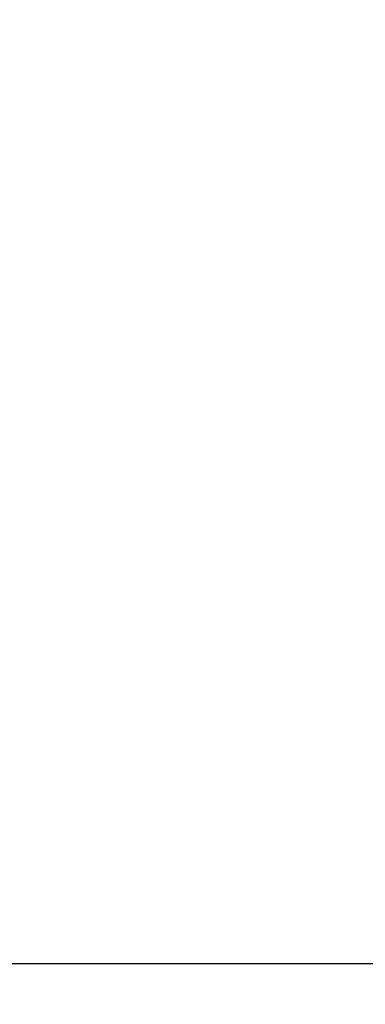
# Model space of a CAD drawing. Units: millimetres. Extents: x 0 to 2267, y 0 to 1823.
# Tile 8 of 256: x 1482.26 to 1490.3, y 1116.48 to 1139.36. Entities that reach past the tile are written whole.
import ezdxf

# ---------------------------------------------------------------- set-up
doc = ezdxf.new("R2010")
doc.units = ezdxf.units.MM
doc.header["$MEASUREMENT"] = 0
doc.layers.add('M-DIMS', color=2, linetype='Continuous', lineweight=25)
doc.layers.add('M-HATC', color=252, linetype='Continuous', lineweight=18)
doc.styles.get("Standard").update_dxf_attribs({"font": 'arial.ttf'})
doc.dimstyles.get("Standard").update_dxf_attribs({"dimtxt": 7, "dimasz": 4, "dimexe": 0.18, "dimexo": 0.0625, "dimgap": 0.09, "dimtad": 0, "dimdec": 0, "dimzin": 0, "dimdsep": 46, "dimtxsty": 'Standard', "dimcen": 0.09, "dimadec": 0, "dimazin": 0, "dimtfac": 1, "dimtdec": 0, "dimtofl": 0, "dimtmove": 0, "dimatfit": 3, "dimfxl": 1, "dimtolj": 1, "dimtzin": 0, "dimarcsym": 0})

# ---------------------------------------------------------------- blocks, each defined once
blk = doc.blocks.new('*D9')
at = {"layer": 'Defpoints', "color": 0, "transparency": 16777216}
for p in [(1332.087, 1117.417), (1505.929, 1117.417), (1505.929, 1077.417)]:
    blk.add_point(p, dxfattribs=at)
at = {"layer": 'M-DIMS', "color": 0, "lineweight": -2, "transparency": 16777216}
for p, q in [((1505.866, 1117.417), (1331.907, 1117.417)), ((1332.087, 1113.417), (1332.087, 1102.65)), ((1332.087, 1081.417), (1332.087, 1092.184)), ((1505.866, 1077.417), (1331.907, 1077.417))]:
    blk.add_line(p, q, dxfattribs=at)
at = {"layer": 'M-DIMS', "color": 0, "transparency": 16777216}
for points in [[(1331.42, 1113.417), (1332.753, 1113.417), (1332.087, 1117.417)], [(1331.42, 1081.417), (1332.753, 1081.417), (1332.087, 1077.417)]]:
    blk.add_solid(points, dxfattribs=at)
at = {"layer": 'M-DIMS', "color": 0, "transparency": 16777216, "insert": (1332.087, 1097.417), "char_height": 7, "attachment_point": 5, "rotation": 90}
blk.add_mtext('\\A1;40', dxfattribs=at)
blk = doc.blocks.new('*D10')
at = {"layer": 'Defpoints', "color": 0, "transparency": 16777216}
for p in [(1332.087, 1287.766), (1505.929, 1287.766), (1505.929, 1117.417)]:
    blk.add_point(p, dxfattribs=at)
at = {"layer": 'M-DIMS', "color": 0, "lineweight": -2, "transparency": 16777216}
for p, q in [((1505.866, 1287.766), (1331.907, 1287.766)), ((1332.087, 1283.766), (1332.087, 1216.908)), ((1332.087, 1121.417), (1332.087, 1188.275)), ((1505.866, 1117.417), (1331.907, 1117.417))]:
    blk.add_line(p, q, dxfattribs=at)
at = {"layer": 'M-DIMS', "color": 0, "transparency": 16777216}
for points in [[(1331.42, 1283.766), (1332.753, 1283.766), (1332.087, 1287.766)], [(1331.42, 1121.417), (1332.753, 1121.417), (1332.087, 1117.417)]]:
    blk.add_solid(points, dxfattribs=at)
at = {"layer": 'M-DIMS', "color": 0, "transparency": 16777216, "insert": (1332.087, 1202.591), "char_height": 7, "attachment_point": 5, "rotation": 90}
blk.add_mtext('\\A1;170.35', dxfattribs=at)

msp = doc.modelspace()

# ---------------------------------------------------------------- hatches: boundary and pattern name
at = {"layer": 'M-HATC'}
h = msp.add_hatch(color=256, dxfattribs=at)
h.dxf.hatch_style = 1
h.paths.add_polyline_path([(2055.771, 1603.062), (1381.087, 1603.062), (1381.087, 1598.062), (2055.771, 1598.062)])
h.paths.add_polyline_path([(2055.771, 1598.062), (1381.087, 1598.062), (1381.087, 1593.062), (2055.771, 1593.062)])
h.paths.add_polyline_path([(2051.307, 1536.761), (1385.55, 1536.761), (1385.55, 1526.761), (1387.55, 1526.761), (1388.537, 1525.053), (1385.332, 1521.233), (1385.332, 1521.223), (2050.254, 1522.749), (2048.321, 1525.053), (2049.307, 1526.761), (2051.307, 1526.761)])
edge = h.paths.add_edge_path()
edge.add_arc((1847.535, 1379.149), 135, 222.60306, 222.89085, ccw=False)
edge.add_line((1748.166, 1287.766), (1683.092, 1287.766))
edge.add_arc((1583.724, 1379.149), 135, 317.10915, 317.39694, ccw=False)
edge.add_arc((1678.969, 1290.671), 5, 222.8909, 317.1091, ccw=False)
edge.add_arc((1774.213, 1379.149), 135, 222.60306, 222.89085, ccw=False)
edge.add_line((1674.845, 1287.766), (1609.771, 1287.766))
edge.add_arc((1510.403, 1379.149), 135, 317.10915, 317.39694, ccw=False)
edge.add_arc((1605.647, 1290.671), 5, 222.8909, 317.1091, ccw=False)
edge.add_arc((1700.892, 1379.149), 135, 222.60306, 222.89085, ccw=False)
edge.add_line((1601.524, 1287.766), (1536.45, 1287.766))
edge.add_arc((1437.081, 1379.149), 135, 317.10915, 317.39694, ccw=False)
edge.add_arc((1532.326, 1290.671), 5, 222.8909, 317.1091, ccw=False)
edge.add_arc((1627.571, 1379.149), 135, 222.60306, 222.89085, ccw=False)
edge.add_line((1528.203, 1287.766), (1505.929, 1287.766))
edge.add_spline(control_points=[(1505.929, 1287.766), (1504.262, 1287.766), (1504.262, 1282.766), (1505.929, 1282.766)], knot_values=[0, 0, 0, 0, 5, 5, 5, 5], degree=3, periodic=0)
edge.add_line((1505.929, 1282.766), (1930.929, 1282.766))
edge.add_spline(control_points=[(1930.929, 1282.766), (1932.596, 1282.766), (1932.596, 1287.766), (1930.929, 1287.766)], knot_values=[0, 0, 0, 0, 5, 5, 5, 5], degree=3, periodic=0)
edge.add_line((1930.929, 1287.766), (1903.056, 1287.766))
edge.add_arc((1803.688, 1379.149), 135, 317.10915, 317.39694, ccw=False)
edge.add_arc((1898.932, 1290.671), 5, 222.8909, 317.1091, ccw=False)
edge.add_arc((1994.177, 1379.149), 135, 222.60306, 222.89085, ccw=False)
edge.add_line((1894.809, 1287.766), (1829.735, 1287.766))
edge.add_arc((1730.366, 1379.149), 135, 317.10915, 317.39694, ccw=False)
edge.add_arc((1825.611, 1290.671), 5, 222.8909, 317.1091, ccw=False)
edge.add_arc((1920.856, 1379.149), 135, 222.60306, 222.89085, ccw=False)
edge.add_line((1821.487, 1287.766), (1756.413, 1287.766))
edge.add_arc((1657.045, 1379.149), 135, 317.10915, 317.39694, ccw=False)
edge.add_arc((1752.29, 1290.671), 5, 222.8909, 317.1091, ccw=False)
edge = h.paths.add_edge_path()
edge.add_spline(control_points=[(1843.429, 1227.247), (1845.096, 1227.247), (1845.096, 1232.247), (1843.429, 1232.247)], knot_values=[0, 0, 0, 0, 5, 5, 5, 5], degree=3, periodic=0)
edge.add_line((1843.429, 1232.247), (1593.429, 1232.247))
edge.add_spline(control_points=[(1593.429, 1232.247), (1591.762, 1232.247), (1591.762, 1227.247), (1593.429, 1227.247)], knot_values=[0, 0, 0, 0, 5, 5, 5, 5], degree=3, periodic=0)
edge.add_line((1593.429, 1227.247), (1843.429, 1227.247))
h.paths.add_polyline_path([(1905.929, 1127.417), (1530.929, 1127.417, 0.414214), (1520.929, 1117.417), (1530.929, 1117.417), (1915.929, 1117.417, 0.414214)])
edge = h.paths.add_edge_path()
edge.add_arc((1397.086, 1498.408), 12.73, 90.7821, 190.8787, ccw=False)
edge.add_line((1396.912, 1511.136), (1428.01, 1511.349))
edge.add_line((1428.01, 1511.349), (1433.01, 1511.349))
edge.add_line((1433.01, 1511.349), (1434.439, 1511.349))
edge.add_arc((1419.474, 1498.08), 20, 41.561, 74.0821)
edge.add_line((1424.959, 1517.314), (1399.935, 1517.256))
edge.add_spline(control_points=[(1399.931, 1517.256), (1399.884, 1517.213), (1399.833, 1517.169), (1399.777, 1517.124)], knot_values=[11.567499, 11.567499, 11.567499, 11.567499, 11.814249, 11.814249, 11.814249, 11.814249], degree=3, periodic=0)
edge.add_spline(control_points=[(1399.633, 1517.01), (1399.583, 1516.972), (1399.531, 1516.934), (1399.476, 1516.895)], knot_values=[11.167718, 11.167718, 11.167718, 11.167718, 11.365188, 11.365188, 11.365188, 11.365188], degree=3, periodic=0)
edge.add_spline(control_points=[(1399.34, 1516.8), (1399.151, 1516.672), (1398.938, 1516.538), (1398.704, 1516.399)], knot_values=[10.376405, 10.376405, 10.376405, 10.376405, 11.00994, 11.00994, 11.00994, 11.00994], degree=3, periodic=0)
edge.add_spline(control_points=[(1398.657, 1516.372), (1398.579, 1516.326), (1398.498, 1516.28), (1398.415, 1516.233)], knot_values=[10.125175, 10.125175, 10.125175, 10.125175, 10.334406, 10.334406, 10.334406, 10.334406], degree=3, periodic=0)
edge.add_spline(control_points=[(1398.264, 1516.149), (1398.196, 1516.111), (1398.126, 1516.073), (1398.055, 1516.035)], knot_values=[9.832246, 9.832246, 9.832246, 9.832246, 9.999658, 9.999658, 9.999658, 9.999658], degree=3, periodic=0)
edge.add_spline(control_points=[(1397.999, 1516.005), (1397.731, 1515.862), (1397.446, 1515.717), (1397.147, 1515.571)], knot_values=[9.161808, 9.161808, 9.161808, 9.161808, 9.787769, 9.787769, 9.787769, 9.787769], degree=3, periodic=0)
edge.add_spline(control_points=[(1397.147, 1515.571), (1396.842, 1515.423), (1396.522, 1515.274), (1396.191, 1515.126)], knot_values=[8.524455, 8.524455, 8.524455, 8.524455, 9.161808, 9.161808, 9.161808, 9.161808], degree=3, periodic=0)
edge.add_spline(control_points=[(1396.078, 1515.076), (1395.985, 1515.035), (1395.892, 1514.994), (1395.798, 1514.953)], knot_values=[8.275193, 8.275193, 8.275193, 8.275193, 8.451726, 8.451726, 8.451726, 8.451726], degree=3, periodic=0)
edge.add_spline(control_points=[(1395.602, 1514.869), (1395.5, 1514.826), (1395.397, 1514.782), (1395.293, 1514.739)], knot_values=[7.962917, 7.962917, 7.962917, 7.962917, 8.152764, 8.152764, 8.152764, 8.152764], degree=3, periodic=0)
edge.add_spline(control_points=[(1395.212, 1514.706), (1394.828, 1514.547), (1394.435, 1514.393), (1394.036, 1514.244)], knot_values=[7.21254, 7.21254, 7.21254, 7.21254, 7.913148, 7.913148, 7.913148, 7.913148], degree=3, periodic=0)
edge.add_spline(control_points=[(1394.036, 1514.244), (1393.708, 1514.121), (1393.375, 1514.003), (1393.043, 1513.889)], knot_values=[6.633733, 6.633733, 6.633733, 6.633733, 7.21254, 7.21254, 7.21254, 7.21254], degree=3, periodic=0)
edge.add_spline(control_points=[(1392.821, 1513.815), (1392.72, 1513.781), (1392.618, 1513.748), (1392.517, 1513.715)], knot_values=[6.328796, 6.328796, 6.328796, 6.328796, 6.505493, 6.505493, 6.505493, 6.505493], degree=3, periodic=0)
edge.add_spline(control_points=[(1392.517, 1513.715), (1392.319, 1513.652), (1392.121, 1513.59), (1391.924, 1513.531)], knot_values=[5.984605, 5.984605, 5.984605, 5.984605, 6.328796, 6.328796, 6.328796, 6.328796], degree=3, periodic=0)
edge.add_spline(control_points=[(1391.792, 1513.491), (1391.312, 1513.35), (1390.838, 1513.224), (1390.378, 1513.117)], knot_values=[5.066697, 5.066697, 5.066697, 5.066697, 5.907055, 5.907055, 5.907055, 5.907055], degree=3, periodic=0)
edge.add_spline(control_points=[(1390.378, 1513.117), (1390.18, 1513.071), (1389.984, 1513.028), (1389.791, 1512.99)], knot_values=[4.70367, 4.70367, 4.70367, 4.70367, 5.066695, 5.066695, 5.066695, 5.066695], degree=3, periodic=0)
edge.add_spline(control_points=[(1389.422, 1512.92), (1389.246, 1512.889), (1389.073, 1512.862), (1388.904, 1512.838)], knot_values=[4.130571, 4.130571, 4.130571, 4.130571, 4.469816, 4.469816, 4.469816, 4.469816], degree=3, periodic=0)
edge.add_spline(control_points=[(1388.904, 1512.838), (1388.591, 1512.795), (1388.291, 1512.764), (1388.007, 1512.749)], knot_values=[3.504031, 3.504031, 3.504031, 3.504031, 4.130571, 4.130571, 4.130571, 4.130571], degree=3, periodic=0)
edge.add_spline(control_points=[(1387.936, 1512.746), (1387.854, 1512.742), (1387.773, 1512.74), (1387.694, 1512.739)], knot_values=[3.268866, 3.268866, 3.268866, 3.268866, 3.451164, 3.451164, 3.451164, 3.451164], degree=3, periodic=0)
edge.add_spline(control_points=[(1387.335, 1512.744), (1387.208, 1512.75), (1387.085, 1512.76), (1386.967, 1512.774)], knot_values=[2.670686, 2.670686, 2.670686, 2.670686, 2.984, 2.984, 2.984, 2.984], degree=3, periodic=0)
edge.add_spline(control_points=[(1386.833, 1512.792), (1386.821, 1512.794), (1386.809, 1512.796), (1386.797, 1512.798)], knot_values=[2.516981, 2.516981, 2.516981, 2.516981, 2.549528, 2.549528, 2.549528, 2.549528], degree=3, periodic=0)
edge.add_spline(control_points=[(1386.453, 1512.873), (1386.426, 1512.881), (1386.399, 1512.889), (1386.373, 1512.897)], knot_values=[2.095869, 2.095869, 2.095869, 2.095869, 2.17941, 2.17941, 2.17941, 2.17941], degree=3, periodic=0)
edge.add_spline(control_points=[(1386.069, 1513.019), (1386.063, 1513.022), (1386.058, 1513.025), (1386.052, 1513.028)], knot_values=[1.72453, 1.72453, 1.72453, 1.72453, 1.745933, 1.745933, 1.745933, 1.745933], degree=3, periodic=0)
edge.add_arc((1399.474, 1498.08), 20, 131.8243, 180)
edge.add_arc((1630.334, 1505.548), 250.971, 181.70518, 236.42798)
edge.add_arc((1605.34, 1483.304), 218.782, 238.66083, 243.34961)
edge.add_arc((1647.091, 1510.359), 262.899, 183.12984, 237.85344, ccw=False)
h.paths.add_polyline_path([(1406.537, 1391.964, 0.149382), (1491.551, 1296.442, -0.129517)], flags=17)
edge = h.paths.add_edge_path()
edge.add_arc((2037.384, 1498.08), 20, 0, 48.2659)
edge.add_spline(control_points=[(2050.697, 1513.005), (2050.651, 1512.985), (2050.603, 1512.966), (2050.554, 1512.948)], knot_values=[1.835652, 1.835652, 1.835652, 1.835652, 2.000781, 2.000781, 2.000781, 2.000781], degree=3, periodic=0)
edge.add_spline(control_points=[(2050.462, 1512.917), (2050.479, 1512.922), (2050.496, 1512.928), (2050.513, 1512.934)], knot_values=[2.045477, 2.045477, 2.045477, 2.045477, 2.101389, 2.101389, 2.101389, 2.101389], degree=3, periodic=0)
edge.add_spline(control_points=[(2050.129, 1512.834), (2050.198, 1512.847), (2050.266, 1512.862), (2050.331, 1512.879)], knot_values=[2.237629, 2.237629, 2.237629, 2.237629, 2.435841, 2.435841, 2.435841, 2.435841], degree=3, periodic=0)
edge.add_spline(control_points=[(2050.095, 1512.828), (2050.106, 1512.83), (2050.118, 1512.832), (2050.129, 1512.834)], knot_values=[2.435841, 2.435841, 2.435841, 2.435841, 2.468321, 2.468321, 2.468321, 2.468321], degree=3, periodic=0)
edge.add_spline(control_points=[(2049.784, 1512.785), (2049.855, 1512.792), (2049.924, 1512.801), (2049.992, 1512.811)], knot_values=[2.563852, 2.563852, 2.563852, 2.563852, 2.748541, 2.748541, 2.748541, 2.748541], degree=3, periodic=0)
edge.add_spline(control_points=[(2049.405, 1512.762), (2049.536, 1512.765), (2049.663, 1512.773), (2049.784, 1512.785)], knot_values=[2.748541, 2.748541, 2.748541, 2.748541, 3.064882, 3.064882, 3.064882, 3.064882], degree=3, periodic=0)
edge.add_spline(control_points=[(2049.17, 1512.76), (2049.234, 1512.759), (2049.297, 1512.759), (2049.358, 1512.761)], knot_values=[3.102309, 3.102309, 3.102309, 3.102309, 3.2503, 3.2503, 3.2503, 3.2503], degree=3, periodic=0)
edge.add_spline(control_points=[(2048.857, 1512.769), (2048.964, 1512.764), (2049.068, 1512.761), (2049.17, 1512.76)], knot_values=[3.2503, 3.2503, 3.2503, 3.2503, 3.486069, 3.486069, 3.486069, 3.486069], degree=3, periodic=0)
edge.add_spline(control_points=[(2048.692, 1512.779), (2048.373, 1512.801), (2048.035, 1512.841), (2047.682, 1512.897)], knot_values=[3.606429, 3.606429, 3.606429, 3.606429, 4.2989, 4.2989, 4.2989, 4.2989], degree=3, periodic=0)
edge.add_spline(control_points=[(2047.682, 1512.897), (2047.546, 1512.919), (2047.408, 1512.942), (2047.268, 1512.969)], knot_values=[4.2989, 4.2989, 4.2989, 4.2989, 4.565769, 4.565769, 4.565769, 4.565769], degree=3, periodic=0)
edge.add_spline(control_points=[(2047.268, 1512.969), (2047.145, 1512.991), (2047.021, 1513.016), (2046.895, 1513.042)], knot_values=[4.565769, 4.565769, 4.565769, 4.565769, 4.799971, 4.799971, 4.799971, 4.799971], degree=3, periodic=0)
edge.add_spline(control_points=[(2046.895, 1513.042), (2046.529, 1513.119), (2046.151, 1513.209), (2045.768, 1513.311)], knot_values=[4.799971, 4.799971, 4.799971, 4.799971, 5.483718, 5.483718, 5.483718, 5.483718], degree=3, periodic=0)
edge.add_spline(control_points=[(2045.768, 1513.311), (2045.372, 1513.415), (2044.97, 1513.532), (2044.566, 1513.659)], knot_values=[5.483718, 5.483718, 5.483718, 5.483718, 6.187866, 6.187866, 6.187866, 6.187866], degree=3, periodic=0)
edge.add_spline(control_points=[(2044.566, 1513.659), (2044.415, 1513.706), (2044.263, 1513.755), (2044.112, 1513.805)], knot_values=[6.187866, 6.187866, 6.187866, 6.187866, 6.451551, 6.451551, 6.451551, 6.451551], degree=3, periodic=0)
edge.add_spline(control_points=[(2044.112, 1513.805), (2043.997, 1513.843), (2043.882, 1513.881), (2043.767, 1513.92)], knot_values=[6.451551, 6.451551, 6.451551, 6.451551, 6.651434, 6.651434, 6.651434, 6.651434], degree=3, periodic=0)
edge.add_spline(control_points=[(2043.767, 1513.92), (2043.372, 1514.055), (2042.977, 1514.198), (2042.589, 1514.346)], knot_values=[6.651434, 6.651434, 6.651434, 6.651434, 7.338879, 7.338879, 7.338879, 7.338879], degree=3, periodic=0)
edge.add_spline(control_points=[(2042.589, 1514.346), (2042.164, 1514.507), (2041.746, 1514.675), (2041.341, 1514.846)], knot_values=[7.338879, 7.338879, 7.338879, 7.338879, 8.089209, 8.089209, 8.089209, 8.089209], degree=3, periodic=0)
edge.add_spline(control_points=[(2041.341, 1514.846), (2041.103, 1514.946), (2040.869, 1515.048), (2040.64, 1515.15)], knot_values=[8.089209, 8.089209, 8.089209, 8.089209, 8.529587, 8.529587, 8.529587, 8.529587], degree=3, periodic=0)
edge.add_spline(control_points=[(2040.51, 1515.209), (2040.082, 1515.402), (2039.675, 1515.597), (2039.295, 1515.789)], knot_values=[8.613818, 8.613818, 8.613818, 8.613818, 9.44571, 9.44571, 9.44571, 9.44571], degree=3, periodic=0)
edge.add_spline(control_points=[(2039.295, 1515.789), (2039.062, 1515.907), (2038.839, 1516.025), (2038.629, 1516.14)], knot_values=[9.44571, 9.44571, 9.44571, 9.44571, 9.956404, 9.956404, 9.956404, 9.956404], degree=3, periodic=0)
edge.add_spline(control_points=[(2038.629, 1516.14), (2038.519, 1516.2), (2038.412, 1516.26), (2038.309, 1516.319)], knot_values=[9.956404, 9.956404, 9.956404, 9.956404, 10.223542, 10.223542, 10.223542, 10.223542], degree=3, periodic=0)
edge.add_spline(control_points=[(2038.309, 1516.319), (2038.214, 1516.374), (2038.122, 1516.428), (2038.033, 1516.481)], knot_values=[10.223542, 10.223542, 10.223542, 10.223542, 10.47051, 10.47051, 10.47051, 10.47051], degree=3, periodic=0)
edge.add_spline(control_points=[(2038.033, 1516.481), (2037.786, 1516.63), (2037.564, 1516.773), (2037.372, 1516.909)], knot_values=[10.47051, 10.47051, 10.47051, 10.47051, 11.15767, 11.15767, 11.15767, 11.15767], degree=3, periodic=0)
edge.add_spline(control_points=[(2037.372, 1516.909), (2037.279, 1516.975), (2037.193, 1517.04), (2037.114, 1517.102)], knot_values=[11.15767, 11.15767, 11.15767, 11.15767, 11.49227, 11.49227, 11.49227, 11.49227], degree=3, periodic=0)
edge.add_spline(control_points=[(2036.856, 1517.326), (2036.915, 1517.269), (2036.981, 1517.21), (2037.056, 1517.149)], knot_values=[11.577341, 11.577341, 11.577341, 11.577341, 11.91035, 11.91035, 11.91035, 11.91035], degree=3, periodic=0)
edge.add_spline(control_points=[(2036.807, 1517.375), (2036.823, 1517.359), (2036.839, 1517.342), (2036.856, 1517.326)], knot_values=[11.91035, 11.91035, 11.91035, 11.91035, 12.007402, 12.007402, 12.007402, 12.007402], degree=3, periodic=0)
edge.add_spline(control_points=[(2036.702, 1517.494), (2036.71, 1517.483), (2036.72, 1517.472), (2036.729, 1517.461)], knot_values=[12.184155, 12.184155, 12.184155, 12.184155, 12.255409, 12.255409, 12.255409, 12.255409], degree=3, periodic=0)
edge.add_spline(control_points=[(2036.616, 1517.621), (2036.62, 1517.613), (2036.624, 1517.606), (2036.629, 1517.598)], knot_values=[12.487913, 12.487913, 12.487913, 12.487913, 12.541035, 12.541035, 12.541035, 12.541035], degree=3, periodic=0)
edge.add_spline(control_points=[(2036.563, 1517.786), (2036.564, 1517.779), (2036.564, 1517.773), (2036.565, 1517.766)], knot_values=[12.911761, 12.911761, 12.911761, 12.911761, 12.968286, 12.968286, 12.968286, 12.968286], degree=3, periodic=0)
edge.add_spline(control_points=[(2036.617, 1517.93), (2036.612, 1517.926), (2036.609, 1517.921), (2036.605, 1517.916)], knot_values=[13.382527, 13.382527, 13.382527, 13.382527, 13.433791, 13.433791, 13.433791, 13.433791], degree=3, periodic=0)
edge.add_spline(control_points=[(2036.749, 1518.017), (2036.736, 1518.012), (2036.724, 1518.006), (2036.712, 1518)], knot_values=[13.726299, 13.726299, 13.726299, 13.726299, 13.809928, 13.809928, 13.809928, 13.809928], degree=3, periodic=0)
edge.add_spline(control_points=[(2036.86, 1518.053), (2036.839, 1518.047), (2036.818, 1518.042), (2036.799, 1518.035)], knot_values=[13.910887, 13.910887, 13.910887, 13.910887, 14.02153, 14.02153, 14.02153, 14.02153], degree=3, periodic=0)
edge.add_line((2036.964, 1518.08), (2032.384, 1518.08))
edge.add_line((2032.384, 1518.08), (2027.384, 1518.08))
edge.add_line((2027.384, 1518.08), (2022.384, 1518.08))
edge.add_line((2022.384, 1518.08), (2017.384, 1518.08))
edge.add_arc((2017.384, 1498.08), 20, 90, 138.439)
edge.add_line((2002.419, 1511.349), (2003.848, 1511.349))
edge.add_line((2003.848, 1511.349), (2008.848, 1511.349))
edge.add_line((2008.848, 1511.349), (2039.772, 1511.138))
edge.add_arc((2039.772, 1498.408), 12.73, -10.8787, 90, ccw=False)
edge.add_arc((1789.767, 1510.359), 262.899, 302.14656, 356.87016, ccw=False)
edge.add_arc((1831.518, 1483.304), 218.782, 296.65039, 301.33917)
edge.add_arc((1806.524, 1505.548), 250.971, 303.57202, 358.29482)
h.paths.add_polyline_path([(2030.321, 1391.964, -0.129517), (1945.307, 1296.442, 0.149382)], flags=17)
edge = h.paths.add_edge_path()
edge.add_spline(control_points=[(2037.246, 1518.082), (2037.29, 1518.081), (2037.336, 1518.08), (2037.384, 1518.08)], knot_values=[0.000012, 0.000012, 0.000012, 0.000012, 0.144754, 0.144754, 0.144754, 0.144754], degree=3, periodic=0)
edge.add_line((2037.336, 1518.08), (2037.01, 1518.08))
edge.add_spline(control_points=[(2037.01, 1518.08), (2036.982, 1518.077), (2036.956, 1518.073), (2036.931, 1518.068)], knot_values=[14.13465, 14.13465, 14.13465, 14.13465, 14.247197, 14.247197, 14.247197, 14.247197], degree=3, periodic=0)
edge.add_spline(control_points=[(2036.931, 1518.068), (2036.928, 1518.067), (2036.924, 1518.067), (2036.921, 1518.066)], knot_values=[14.118315, 14.118315, 14.118315, 14.118315, 14.13465, 14.13465, 14.13465, 14.13465], degree=3, periodic=0)
edge.add_spline(control_points=[(2036.921, 1518.066), (2036.912, 1518.064), (2036.903, 1518.063), (2036.895, 1518.061)], knot_values=[14.078086, 14.078086, 14.078086, 14.078086, 14.118315, 14.118315, 14.118315, 14.118315], degree=3, periodic=0)
edge.add_spline(control_points=[(2036.895, 1518.061), (2036.883, 1518.058), (2036.872, 1518.056), (2036.86, 1518.053)], knot_values=[14.02153, 14.02153, 14.02153, 14.02153, 14.078086, 14.078086, 14.078086, 14.078086], degree=3, periodic=0)
edge.add_spline(control_points=[(2036.86, 1518.053), (2036.839, 1518.047), (2036.818, 1518.042), (2036.799, 1518.035)], knot_values=[13.910887, 13.910887, 13.910887, 13.910887, 14.02153, 14.02153, 14.02153, 14.02153], degree=3, periodic=0)
edge.add_spline(control_points=[(2036.799, 1518.035), (2036.798, 1518.035), (2036.797, 1518.035), (2036.797, 1518.035)], knot_values=[13.906906, 13.906906, 13.906906, 13.906906, 13.910887, 13.910887, 13.910887, 13.910887], degree=3, periodic=0)
edge.add_spline(control_points=[(2036.797, 1518.035), (2036.788, 1518.032), (2036.78, 1518.029), (2036.772, 1518.026)], knot_values=[13.857826, 13.857826, 13.857826, 13.857826, 13.906906, 13.906906, 13.906906, 13.906906], degree=3, periodic=0)
edge.add_spline(control_points=[(2036.772, 1518.026), (2036.764, 1518.023), (2036.756, 1518.02), (2036.749, 1518.017)], knot_values=[13.809928, 13.809928, 13.809928, 13.809928, 13.857826, 13.857826, 13.857826, 13.857826], degree=3, periodic=0)
edge.add_spline(control_points=[(2036.749, 1518.017), (2036.736, 1518.012), (2036.724, 1518.006), (2036.712, 1518)], knot_values=[13.726299, 13.726299, 13.726299, 13.726299, 13.809928, 13.809928, 13.809928, 13.809928], degree=3, periodic=0)
edge.add_spline(control_points=[(2036.712, 1518), (2036.712, 1518), (2036.712, 1518), (2036.711, 1518)], knot_values=[13.723993, 13.723993, 13.723993, 13.723993, 13.726299, 13.726299, 13.726299, 13.726299], degree=3, periodic=0)
edge.add_spline(control_points=[(2036.711, 1518), (2036.706, 1517.997), (2036.701, 1517.994), (2036.696, 1517.992)], knot_values=[13.686536, 13.686536, 13.686536, 13.686536, 13.723993, 13.723993, 13.723993, 13.723993], degree=3, periodic=0)
edge.add_spline(control_points=[(2036.696, 1517.992), (2036.692, 1517.989), (2036.687, 1517.987), (2036.683, 1517.984)], knot_values=[13.651251, 13.651251, 13.651251, 13.651251, 13.686536, 13.686536, 13.686536, 13.686536], degree=3, periodic=0)
edge.add_spline(control_points=[(2036.683, 1517.984), (2036.676, 1517.98), (2036.67, 1517.976), (2036.664, 1517.971)], knot_values=[13.596804, 13.596804, 13.596804, 13.596804, 13.651251, 13.651251, 13.651251, 13.651251], degree=3, periodic=0)
edge.add_spline(control_points=[(2036.664, 1517.971), (2036.664, 1517.971), (2036.663, 1517.971), (2036.663, 1517.971)], knot_values=[13.593956, 13.593956, 13.593956, 13.593956, 13.596804, 13.596804, 13.596804, 13.596804], degree=3, periodic=0)
edge.add_spline(control_points=[(2036.663, 1517.971), (2036.66, 1517.969), (2036.658, 1517.967), (2036.655, 1517.965)], knot_values=[13.570322, 13.570322, 13.570322, 13.570322, 13.593956, 13.593956, 13.593956, 13.593956], degree=3, periodic=0)
edge.add_spline(control_points=[(2036.655, 1517.965), (2036.653, 1517.963), (2036.65, 1517.961), (2036.647, 1517.959)], knot_values=[13.545477, 13.545477, 13.545477, 13.545477, 13.570322, 13.570322, 13.570322, 13.570322], degree=3, periodic=0)
edge.add_spline(control_points=[(2036.647, 1517.959), (2036.647, 1517.959), (2036.647, 1517.959), (2036.647, 1517.959)], knot_values=[13.543931, 13.543931, 13.543931, 13.543931, 13.545477, 13.545477, 13.545477, 13.545477], degree=3, periodic=0)
edge.add_spline(control_points=[(2036.647, 1517.959), (2036.641, 1517.954), (2036.636, 1517.949), (2036.631, 1517.945)], knot_values=[13.488237, 13.488237, 13.488237, 13.488237, 13.543931, 13.543931, 13.543931, 13.543931], degree=3, periodic=0)
edge.add_spline(control_points=[(2036.631, 1517.945), (2036.628, 1517.942), (2036.626, 1517.94), (2036.623, 1517.937)], knot_values=[13.460307, 13.460307, 13.460307, 13.460307, 13.488237, 13.488237, 13.488237, 13.488237], degree=3, periodic=0)
edge.add_spline(control_points=[(2036.623, 1517.937), (2036.622, 1517.936), (2036.62, 1517.934), (2036.618, 1517.932)], knot_values=[13.439712, 13.439712, 13.439712, 13.439712, 13.460307, 13.460307, 13.460307, 13.460307], degree=3, periodic=0)
edge.add_spline(control_points=[(2036.618, 1517.932), (2036.618, 1517.931), (2036.617, 1517.931), (2036.617, 1517.93)], knot_values=[13.433791, 13.433791, 13.433791, 13.433791, 13.439712, 13.439712, 13.439712, 13.439712], degree=3, periodic=0)
edge.add_spline(control_points=[(2036.617, 1517.93), (2036.612, 1517.926), (2036.609, 1517.921), (2036.605, 1517.916)], knot_values=[13.382527, 13.382527, 13.382527, 13.382527, 13.433791, 13.433791, 13.433791, 13.433791], degree=3, periodic=0)
edge.add_spline(control_points=[(2036.605, 1517.916), (2036.603, 1517.913), (2036.6, 1517.91), (2036.598, 1517.907)], knot_values=[13.350017, 13.350017, 13.350017, 13.350017, 13.382527, 13.382527, 13.382527, 13.382527], degree=3, periodic=0)
edge.add_spline(control_points=[(2036.598, 1517.907), (2036.597, 1517.906), (2036.596, 1517.904), (2036.595, 1517.903)], knot_values=[13.333922, 13.333922, 13.333922, 13.333922, 13.350017, 13.350017, 13.350017, 13.350017], degree=3, periodic=0)
edge.add_spline(control_points=[(2036.595, 1517.903), (2036.595, 1517.902), (2036.594, 1517.901), (2036.593, 1517.9)], knot_values=[13.323828, 13.323828, 13.323828, 13.323828, 13.333922, 13.333922, 13.333922, 13.333922], degree=3, periodic=0)
edge.add_spline(control_points=[(2036.593, 1517.9), (2036.59, 1517.895), (2036.588, 1517.891), (2036.585, 1517.886)], knot_values=[13.277545, 13.277545, 13.277545, 13.277545, 13.323828, 13.323828, 13.323828, 13.323828], degree=3, periodic=0)
edge.add_spline(control_points=[(2036.585, 1517.886), (2036.584, 1517.883), (2036.582, 1517.879), (2036.58, 1517.875)], knot_values=[13.240119, 13.240119, 13.240119, 13.240119, 13.277545, 13.277545, 13.277545, 13.277545], degree=3, periodic=0)
edge.add_spline(control_points=[(2036.58, 1517.875), (2036.58, 1517.874), (2036.579, 1517.873), (2036.578, 1517.872)], knot_values=[13.228211, 13.228211, 13.228211, 13.228211, 13.240119, 13.240119, 13.240119, 13.240119], degree=3, periodic=0)
edge.add_spline(control_points=[(2036.578, 1517.872), (2036.578, 1517.87), (2036.577, 1517.869), (2036.577, 1517.868)], knot_values=[13.215717, 13.215717, 13.215717, 13.215717, 13.228211, 13.228211, 13.228211, 13.228211], degree=3, periodic=0)
edge.add_spline(control_points=[(2036.577, 1517.868), (2036.575, 1517.864), (2036.574, 1517.86), (2036.573, 1517.857)], knot_values=[13.179847, 13.179847, 13.179847, 13.179847, 13.215717, 13.215717, 13.215717, 13.215717], degree=3, periodic=0)
edge.add_spline(control_points=[(2036.573, 1517.857), (2036.571, 1517.851), (2036.57, 1517.846), (2036.569, 1517.841)], knot_values=[13.132017, 13.132017, 13.132017, 13.132017, 13.179847, 13.179847, 13.179847, 13.179847], degree=3, periodic=0)
edge.add_spline(control_points=[(2036.569, 1517.841), (2036.568, 1517.84), (2036.568, 1517.839), (2036.568, 1517.838)], knot_values=[13.122482, 13.122482, 13.122482, 13.122482, 13.132017, 13.132017, 13.132017, 13.132017], degree=3, periodic=0)
edge.add_spline(control_points=[(2036.568, 1517.838), (2036.568, 1517.836), (2036.567, 1517.835), (2036.567, 1517.833)], knot_values=[13.105592, 13.105592, 13.105592, 13.105592, 13.122482, 13.122482, 13.122482, 13.122482], degree=3, periodic=0)
edge.add_spline(control_points=[(2036.567, 1517.833), (2036.566, 1517.829), (2036.566, 1517.826), (2036.565, 1517.822)], knot_values=[13.074063, 13.074063, 13.074063, 13.074063, 13.105592, 13.105592, 13.105592, 13.105592], degree=3, periodic=0)
edge.add_spline(control_points=[(2036.565, 1517.822), (2036.565, 1517.822), (2036.565, 1517.822), (2036.565, 1517.822)], knot_values=[13.074043, 13.074043, 13.074043, 13.074043, 13.074063, 13.074063, 13.074063, 13.074063], degree=3, periodic=0)
edge.add_spline(control_points=[(2036.565, 1517.822), (2036.564, 1517.816), (2036.564, 1517.811), (2036.564, 1517.805)], knot_values=[13.021884, 13.021884, 13.021884, 13.021884, 13.074043, 13.074043, 13.074043, 13.074043], degree=3, periodic=0)
edge.add_spline(control_points=[(2036.564, 1517.805), (2036.564, 1517.804), (2036.564, 1517.803), (2036.564, 1517.803)], knot_values=[13.01674, 13.01674, 13.01674, 13.01674, 13.021884, 13.021884, 13.021884, 13.021884], degree=3, periodic=0)
edge.add_spline(control_points=[(2036.564, 1517.803), (2036.563, 1517.801), (2036.563, 1517.798), (2036.563, 1517.796)], knot_values=[12.996438, 12.996438, 12.996438, 12.996438, 13.01674, 13.01674, 13.01674, 13.01674], degree=3, periodic=0)
edge.add_spline(control_points=[(2036.563, 1517.796), (2036.563, 1517.793), (2036.563, 1517.789), (2036.563, 1517.786)], knot_values=[12.968286, 12.968286, 12.968286, 12.968286, 12.996438, 12.996438, 12.996438, 12.996438], degree=3, periodic=0)
edge.add_spline(control_points=[(2036.563, 1517.786), (2036.564, 1517.779), (2036.564, 1517.773), (2036.565, 1517.766)], knot_values=[12.911761, 12.911761, 12.911761, 12.911761, 12.968286, 12.968286, 12.968286, 12.968286], degree=3, periodic=0)
edge.add_spline(control_points=[(2036.565, 1517.766), (2036.565, 1517.766), (2036.565, 1517.766), (2036.565, 1517.766)], knot_values=[12.911017, 12.911017, 12.911017, 12.911017, 12.911761, 12.911761, 12.911761, 12.911761], degree=3, periodic=0)
edge.add_spline(control_points=[(2036.565, 1517.766), (2036.565, 1517.762), (2036.566, 1517.759), (2036.566, 1517.756)], knot_values=[12.88528, 12.88528, 12.88528, 12.88528, 12.911017, 12.911017, 12.911017, 12.911017], degree=3, periodic=0)
edge.add_spline(control_points=[(2036.566, 1517.756), (2036.567, 1517.753), (2036.567, 1517.751), (2036.568, 1517.748)], knot_values=[12.862519, 12.862519, 12.862519, 12.862519, 12.88528, 12.88528, 12.88528, 12.88528], degree=3, periodic=0)
edge.add_spline(control_points=[(2036.568, 1517.748), (2036.568, 1517.747), (2036.568, 1517.747), (2036.568, 1517.746)], knot_values=[12.858885, 12.858885, 12.858885, 12.858885, 12.862519, 12.862519, 12.862519, 12.862519], degree=3, periodic=0)
edge.add_spline(control_points=[(2036.568, 1517.746), (2036.569, 1517.74), (2036.571, 1517.733), (2036.572, 1517.726)], knot_values=[12.8053, 12.8053, 12.8053, 12.8053, 12.858885, 12.858885, 12.858885, 12.858885], degree=3, periodic=0)
edge.add_spline(control_points=[(2036.572, 1517.726), (2036.573, 1517.723), (2036.574, 1517.719), (2036.576, 1517.715)], knot_values=[12.775176, 12.775176, 12.775176, 12.775176, 12.8053, 12.8053, 12.8053, 12.8053], degree=3, periodic=0)
edge.add_spline(control_points=[(2036.576, 1517.715), (2036.576, 1517.713), (2036.577, 1517.71), (2036.578, 1517.708)], knot_values=[12.756759, 12.756759, 12.756759, 12.756759, 12.775176, 12.775176, 12.775176, 12.775176], degree=3, periodic=0)
edge.add_spline(control_points=[(2036.578, 1517.708), (2036.578, 1517.707), (2036.578, 1517.706), (2036.579, 1517.705)], knot_values=[12.748742, 12.748742, 12.748742, 12.748742, 12.756759, 12.756759, 12.756759, 12.756759], degree=3, periodic=0)
edge.add_spline(control_points=[(2036.579, 1517.705), (2036.581, 1517.698), (2036.583, 1517.692), (2036.586, 1517.685)], knot_values=[12.69959, 12.69959, 12.69959, 12.69959, 12.748742, 12.748742, 12.748742, 12.748742], degree=3, periodic=0)
edge.add_spline(control_points=[(2036.586, 1517.685), (2036.588, 1517.68), (2036.59, 1517.675), (2036.592, 1517.669)], knot_values=[12.659038, 12.659038, 12.659038, 12.659038, 12.69959, 12.69959, 12.69959, 12.69959], degree=3, periodic=0)
edge.add_spline(control_points=[(2036.592, 1517.669), (2036.594, 1517.665), (2036.596, 1517.66), (2036.598, 1517.656)], knot_values=[12.626806, 12.626806, 12.626806, 12.626806, 12.659038, 12.659038, 12.659038, 12.659038], degree=3, periodic=0)
edge.add_spline(control_points=[(2036.598, 1517.656), (2036.598, 1517.655), (2036.599, 1517.654), (2036.599, 1517.653)], knot_values=[12.619394, 12.619394, 12.619394, 12.619394, 12.626806, 12.626806, 12.626806, 12.626806], degree=3, periodic=0)
edge.add_spline(control_points=[(2036.599, 1517.653), (2036.604, 1517.642), (2036.61, 1517.632), (2036.616, 1517.621)], knot_values=[12.541039, 12.541039, 12.541039, 12.541039, 12.619394, 12.619394, 12.619394, 12.619394], degree=3, periodic=0)
edge.add_spline(control_points=[(2036.616, 1517.621), (2036.616, 1517.621), (2036.616, 1517.621), (2036.616, 1517.621)], knot_values=[12.541035, 12.541035, 12.541035, 12.541035, 12.541039, 12.541039, 12.541039, 12.541039], degree=3, periodic=0)
edge.add_spline(control_points=[(2036.616, 1517.621), (2036.62, 1517.613), (2036.624, 1517.606), (2036.629, 1517.598)], knot_values=[12.487913, 12.487913, 12.487913, 12.487913, 12.541035, 12.541035, 12.541035, 12.541035], degree=3, periodic=0)
edge.add_spline(control_points=[(2036.629, 1517.598), (2036.633, 1517.592), (2036.637, 1517.585), (2036.641, 1517.579)], knot_values=[12.443982, 12.443982, 12.443982, 12.443982, 12.487913, 12.487913, 12.487913, 12.487913], degree=3, periodic=0)
edge.add_spline(control_points=[(2036.641, 1517.579), (2036.641, 1517.578), (2036.642, 1517.576), (2036.643, 1517.575)], knot_values=[12.434996, 12.434996, 12.434996, 12.434996, 12.443982, 12.443982, 12.443982, 12.443982], degree=3, periodic=0)
edge.add_spline(control_points=[(2036.643, 1517.575), (2036.653, 1517.56), (2036.664, 1517.544), (2036.676, 1517.528)], knot_values=[12.329647, 12.329647, 12.329647, 12.329647, 12.434996, 12.434996, 12.434996, 12.434996], degree=3, periodic=0)
edge.add_spline(control_points=[(2036.676, 1517.528), (2036.684, 1517.517), (2036.693, 1517.505), (2036.702, 1517.494)], knot_values=[12.255409, 12.255409, 12.255409, 12.255409, 12.329647, 12.329647, 12.329647, 12.329647], degree=3, periodic=0)
edge.add_spline(control_points=[(2036.702, 1517.494), (2036.71, 1517.483), (2036.72, 1517.472), (2036.729, 1517.461)], knot_values=[12.184155, 12.184155, 12.184155, 12.184155, 12.255409, 12.255409, 12.255409, 12.255409], degree=3, periodic=0)
edge.add_spline(control_points=[(2036.729, 1517.461), (2036.744, 1517.444), (2036.759, 1517.426), (2036.775, 1517.409)], knot_values=[12.075961, 12.075961, 12.075961, 12.075961, 12.184155, 12.184155, 12.184155, 12.184155], degree=3, periodic=0)
edge.add_spline(control_points=[(2036.775, 1517.409), (2036.776, 1517.407), (2036.777, 1517.406), (2036.778, 1517.405)], knot_values=[12.069502, 12.069502, 12.069502, 12.069502, 12.075961, 12.075961, 12.075961, 12.075961], degree=3, periodic=0)
edge.add_spline(control_points=[(2036.778, 1517.405), (2036.788, 1517.395), (2036.797, 1517.385), (2036.807, 1517.375)], knot_values=[12.007402, 12.007402, 12.007402, 12.007402, 12.069502, 12.069502, 12.069502, 12.069502], degree=3, periodic=0)
edge.add_spline(control_points=[(2036.807, 1517.375), (2036.823, 1517.359), (2036.839, 1517.342), (2036.856, 1517.326)], knot_values=[11.91035, 11.91035, 11.91035, 11.91035, 12.007402, 12.007402, 12.007402, 12.007402], degree=3, periodic=0)
edge.add_spline(control_points=[(2036.856, 1517.326), (2036.915, 1517.269), (2036.981, 1517.21), (2037.056, 1517.149)], knot_values=[11.577341, 11.577341, 11.577341, 11.577341, 11.91035, 11.91035, 11.91035, 11.91035], degree=3, periodic=0)
edge.add_spline(control_points=[(2037.056, 1517.149), (2037.075, 1517.134), (2037.094, 1517.118), (2037.114, 1517.102)], knot_values=[11.49227, 11.49227, 11.49227, 11.49227, 11.577341, 11.577341, 11.577341, 11.577341], degree=3, periodic=0)
edge.add_spline(control_points=[(2037.114, 1517.102), (2037.193, 1517.04), (2037.279, 1516.975), (2037.372, 1516.909)], knot_values=[11.15767, 11.15767, 11.15767, 11.15767, 11.49227, 11.49227, 11.49227, 11.49227], degree=3, periodic=0)
edge.add_spline(control_points=[(2037.372, 1516.909), (2037.564, 1516.773), (2037.786, 1516.63), (2038.033, 1516.481)], knot_values=[10.47051, 10.47051, 10.47051, 10.47051, 11.15767, 11.15767, 11.15767, 11.15767], degree=3, periodic=0)
edge.add_spline(control_points=[(2038.033, 1516.481), (2038.122, 1516.428), (2038.214, 1516.374), (2038.309, 1516.319)], knot_values=[10.223542, 10.223542, 10.223542, 10.223542, 10.47051, 10.47051, 10.47051, 10.47051], degree=3, periodic=0)
edge.add_spline(control_points=[(2038.309, 1516.319), (2038.412, 1516.26), (2038.519, 1516.2), (2038.629, 1516.14)], knot_values=[9.956404, 9.956404, 9.956404, 9.956404, 10.223542, 10.223542, 10.223542, 10.223542], degree=3, periodic=0)
edge.add_spline(control_points=[(2038.629, 1516.14), (2038.839, 1516.025), (2039.062, 1515.907), (2039.295, 1515.789)], knot_values=[9.44571, 9.44571, 9.44571, 9.44571, 9.956404, 9.956404, 9.956404, 9.956404], degree=3, periodic=0)
edge.add_spline(control_points=[(2039.295, 1515.789), (2039.675, 1515.597), (2040.082, 1515.402), (2040.51, 1515.209)], knot_values=[8.613818, 8.613818, 8.613818, 8.613818, 9.44571, 9.44571, 9.44571, 9.44571], degree=3, periodic=0)
edge.add_spline(control_points=[(2040.51, 1515.209), (2040.553, 1515.189), (2040.597, 1515.17), (2040.64, 1515.15)], knot_values=[8.529587, 8.529587, 8.529587, 8.529587, 8.613818, 8.613818, 8.613818, 8.613818], degree=3, periodic=0)
edge.add_spline(control_points=[(2040.64, 1515.15), (2040.869, 1515.048), (2041.103, 1514.946), (2041.341, 1514.846)], knot_values=[8.089209, 8.089209, 8.089209, 8.089209, 8.529587, 8.529587, 8.529587, 8.529587], degree=3, periodic=0)
edge.add_spline(control_points=[(2041.341, 1514.846), (2041.746, 1514.675), (2042.164, 1514.507), (2042.589, 1514.346)], knot_values=[7.338879, 7.338879, 7.338879, 7.338879, 8.089209, 8.089209, 8.089209, 8.089209], degree=3, periodic=0)
edge.add_spline(control_points=[(2042.589, 1514.346), (2042.977, 1514.198), (2043.372, 1514.055), (2043.767, 1513.92)], knot_values=[6.651434, 6.651434, 6.651434, 6.651434, 7.338879, 7.338879, 7.338879, 7.338879], degree=3, periodic=0)
edge.add_spline(control_points=[(2043.767, 1513.92), (2043.882, 1513.881), (2043.997, 1513.843), (2044.112, 1513.805)], knot_values=[6.451551, 6.451551, 6.451551, 6.451551, 6.651434, 6.651434, 6.651434, 6.651434], degree=3, periodic=0)
edge.add_spline(control_points=[(2044.112, 1513.805), (2044.263, 1513.755), (2044.415, 1513.706), (2044.566, 1513.659)], knot_values=[6.187866, 6.187866, 6.187866, 6.187866, 6.451551, 6.451551, 6.451551, 6.451551], degree=3, periodic=0)
edge.add_spline(control_points=[(2044.566, 1513.659), (2044.97, 1513.532), (2045.372, 1513.415), (2045.768, 1513.311)], knot_values=[5.483718, 5.483718, 5.483718, 5.483718, 6.187866, 6.187866, 6.187866, 6.187866], degree=3, periodic=0)
edge.add_spline(control_points=[(2045.768, 1513.311), (2046.151, 1513.209), (2046.529, 1513.119), (2046.895, 1513.042)], knot_values=[4.799971, 4.799971, 4.799971, 4.799971, 5.483718, 5.483718, 5.483718, 5.483718], degree=3, periodic=0)
edge.add_spline(control_points=[(2046.895, 1513.042), (2047.021, 1513.016), (2047.145, 1512.991), (2047.268, 1512.969)], knot_values=[4.565769, 4.565769, 4.565769, 4.565769, 4.799971, 4.799971, 4.799971, 4.799971], degree=3, periodic=0)
edge.add_spline(control_points=[(2047.268, 1512.969), (2047.408, 1512.942), (2047.546, 1512.919), (2047.682, 1512.897)], knot_values=[4.2989, 4.2989, 4.2989, 4.2989, 4.565769, 4.565769, 4.565769, 4.565769], degree=3, periodic=0)
edge.add_spline(control_points=[(2047.682, 1512.897), (2048.035, 1512.841), (2048.373, 1512.801), (2048.692, 1512.779)], knot_values=[3.606429, 3.606429, 3.606429, 3.606429, 4.2989, 4.2989, 4.2989, 4.2989], degree=3, periodic=0)
edge.add_spline(control_points=[(2048.692, 1512.779), (2048.748, 1512.775), (2048.803, 1512.772), (2048.857, 1512.769)], knot_values=[3.486069, 3.486069, 3.486069, 3.486069, 3.606429, 3.606429, 3.606429, 3.606429], degree=3, periodic=0)
edge.add_spline(control_points=[(2048.857, 1512.769), (2048.964, 1512.764), (2049.068, 1512.761), (2049.17, 1512.76)], knot_values=[3.2503, 3.2503, 3.2503, 3.2503, 3.486069, 3.486069, 3.486069, 3.486069], degree=3, periodic=0)
edge.add_spline(control_points=[(2049.17, 1512.76), (2049.234, 1512.759), (2049.297, 1512.759), (2049.358, 1512.761)], knot_values=[3.102309, 3.102309, 3.102309, 3.102309, 3.2503, 3.2503, 3.2503, 3.2503], degree=3, periodic=0)
edge.add_spline(control_points=[(2049.358, 1512.761), (2049.374, 1512.761), (2049.39, 1512.761), (2049.405, 1512.762)], knot_values=[3.064882, 3.064882, 3.064882, 3.064882, 3.102309, 3.102309, 3.102309, 3.102309], degree=3, periodic=0)
edge.add_spline(control_points=[(2049.405, 1512.762), (2049.536, 1512.765), (2049.663, 1512.773), (2049.784, 1512.785)], knot_values=[2.748541, 2.748541, 2.748541, 2.748541, 3.064882, 3.064882, 3.064882, 3.064882], degree=3, periodic=0)
edge.add_spline(control_points=[(2049.784, 1512.785), (2049.855, 1512.792), (2049.924, 1512.801), (2049.992, 1512.811)], knot_values=[2.563852, 2.563852, 2.563852, 2.563852, 2.748541, 2.748541, 2.748541, 2.748541], degree=3, periodic=0)
edge.add_spline(control_points=[(2049.992, 1512.811), (2050.026, 1512.816), (2050.061, 1512.822), (2050.095, 1512.828)], knot_values=[2.468321, 2.468321, 2.468321, 2.468321, 2.563852, 2.563852, 2.563852, 2.563852], degree=3, periodic=0)
edge.add_spline(control_points=[(2050.095, 1512.828), (2050.106, 1512.83), (2050.118, 1512.832), (2050.129, 1512.834)], knot_values=[2.435841, 2.435841, 2.435841, 2.435841, 2.468321, 2.468321, 2.468321, 2.468321], degree=3, periodic=0)
edge.add_spline(control_points=[(2050.129, 1512.834), (2050.198, 1512.847), (2050.266, 1512.862), (2050.331, 1512.879)], knot_values=[2.237629, 2.237629, 2.237629, 2.237629, 2.435841, 2.435841, 2.435841, 2.435841], degree=3, periodic=0)
edge.add_spline(control_points=[(2050.331, 1512.879), (2050.375, 1512.891), (2050.419, 1512.903), (2050.462, 1512.917)], knot_values=[2.101389, 2.101389, 2.101389, 2.101389, 2.237629, 2.237629, 2.237629, 2.237629], degree=3, periodic=0)
edge.add_spline(control_points=[(2050.462, 1512.917), (2050.479, 1512.922), (2050.496, 1512.928), (2050.513, 1512.934)], knot_values=[2.045477, 2.045477, 2.045477, 2.045477, 2.101389, 2.101389, 2.101389, 2.101389], degree=3, periodic=0)
edge.add_spline(control_points=[(2050.513, 1512.934), (2050.527, 1512.938), (2050.54, 1512.943), (2050.554, 1512.948)], knot_values=[2.000781, 2.000781, 2.000781, 2.000781, 2.045477, 2.045477, 2.045477, 2.045477], degree=3, periodic=0)
edge.add_spline(control_points=[(2050.554, 1512.948), (2050.603, 1512.966), (2050.651, 1512.985), (2050.697, 1513.005)], knot_values=[1.835652, 1.835652, 1.835652, 1.835652, 2.000781, 2.000781, 2.000781, 2.000781], degree=3, periodic=0)
edge.add_arc((2037.384, 1498.08), 20, 48.2659, 90.1299)
edge = h.paths.add_edge_path(flags=16)
edge.add_spline(control_points=[(1386.139, 1512.986), (1388.92, 1511.739), (1398.039, 1515.519), (1399.931, 1517.256)], knot_values=[1.831046, 1.831046, 1.831046, 1.831046, 11.814249, 11.814249, 11.814249, 11.814249], degree=3, periodic=0)
edge.add_line((1399.931, 1517.256), (1393.743, 1517.242))
edge.add_arc((1399.474, 1498.08), 20, 106.6501, 131.8173)

# ---------------------------------------------------------------- dimensions: what is measured, and where the dimension line sits
at = {"layer": 'M-DIMS'}
for base, p1, p2, override, picture, middle in [((1332.087, 1287.766), (1505.929, 1117.417), (1505.929, 1287.766), {"dimdec": 2, "dimlfac": 1, "dimrnd": 0, "dimzin": 0, "dimdsep": 46, "dimlunit": 2}, '*D10', (1332.087, 1202.591)), ((1332.087, 1117.417), (1505.929, 1077.417), (1505.929, 1117.417), {"dimdec": 0, "dimlfac": 1, "dimrnd": 0, "dimzin": 0, "dimdsep": 46, "dimlunit": 2}, '*D9', (1332.087, 1097.417))]:
    dim = msp.add_linear_dim(base=base, p1=p1, p2=p2, angle=90, dimstyle='Standard', override=override, dxfattribs=at)
    dim.commit()
    dim.dimension.update_dxf_attribs({"geometry": picture, "text_midpoint": middle})

doc.saveas('drawing.dxf')
